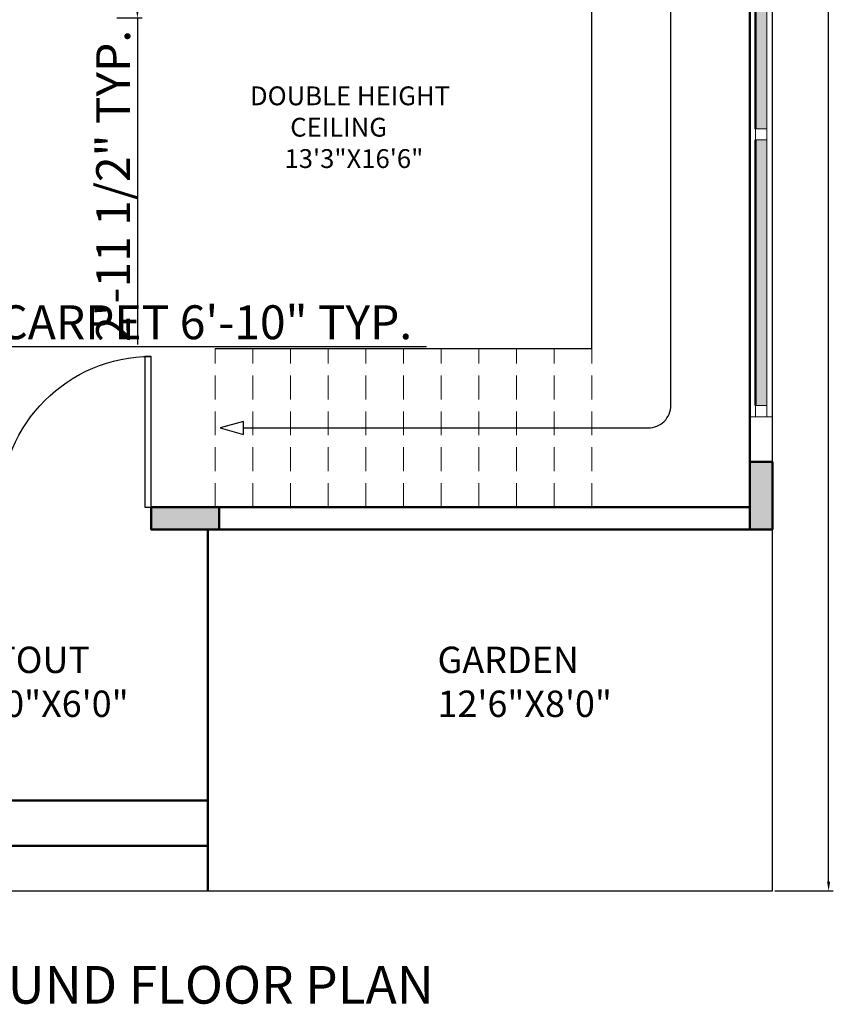
# Model space of a CAD drawing. Units: inches. Extents: x 3064 to 19385, y 846 to 15425.
# Tile 2 of 108: x 3363 to 3579, y 850 to 1112. Entities that reach past the tile are written whole.
import ezdxf

# ---------------------------------------------------------------- set-up
doc = ezdxf.new("R2010")
doc.units = ezdxf.units.IN
doc.linetypes.add('DASHED', pattern=[19.05, 12.7, -6.35])
for name, color, linetype, lineweight in [('A-ANNO-DIMS', 2, 'Continuous', 18), ('A-ANNO-TEXT', 7, 'Continuous', 25), ('A-AREA-IDEN', 3, 'Continuous', 18), ('A-COLS', 1, 'Continuous', 35), ('A-DOOR', 3, 'Continuous', 25), ('A-FLOR-STRS', 2, 'Continuous', 25), ('A-FLOR-STRS-OVHD', 2, 'DASHED', 18), ('A-GLAZ', 4, 'Continuous', 18), ('A-WALL', 7, 'Continuous', 50), ('C-PROP', 6, 'Continuous', 25)]:
    doc.layers.add(name, color=color, linetype=linetype, lineweight=lineweight)
doc.styles.get("Standard").update_dxf_attribs({"font": 'arial.ttf'})
doc.dimstyles.new('ISO-25', dxfattribs={"dimtxt": 9, "dimasz": 2.5, "dimexe": 1.25, "dimexo": 0.625, "dimtad": 1, "dimdec": 1, "dimlunit": 3, "dimtxsty": 'Standard', "dimcen": 2.5, "dimadec": 0, "dimazin": 0, "dimtfac": 1, "dimtdec": 1, "dimtmove": 0, "dimatfit": 3, "dimfxl": 1, "dimarcsym": 0})

# ---------------------------------------------------------------- blocks, each defined once
blk = doc.blocks.new('*U2')
for p, q in [((0, 0), (0, -6)), ((40, 0), (40, -6))]:
    blk.add_line(p, q)
blk.add_lwpolyline([(0, 0), (0, 40), (1.75, 40), (1.75, 0)], close=True)
blk.add_arc((0, 0), 40, 0, 90)
blk = doc.blocks.new('*D42')
at = {"layer": 'A-ANNO-DIMS', "color": 0, "lineweight": -2, "transparency": 16777216}
for p, q in [((3563.47, 1396.34), (3579.02, 1396.34)), ((3577.77, 882.84), (3577.77, 1393.84)), ((3563.47, 880.34), (3579.02, 880.34))]:
    blk.add_line(p, q, dxfattribs=at)
at = {"layer": 'A-ANNO-DIMS', "color": 0, "transparency": 16777216}
for points in [[(3577.35, 1393.84), (3578.19, 1393.84), (3577.77, 1396.34)], [(3577.35, 882.84), (3578.19, 882.84), (3577.77, 880.34)]]:
    blk.add_solid(points, dxfattribs=at)
at = {"layer": 'Defpoints', "color": 0, "transparency": 16777216}
for p in [(3562.85, 1396.34), (3577.77, 1396.34), (3562.85, 880.34)]:
    blk.add_point(p, dxfattribs=at)
at = {"layer": 'A-ANNO-DIMS', "color": 0, "transparency": 16777216, "insert": (3572.55, 1138.34), "char_height": 9, "attachment_point": 5, "rotation": 90}
blk.add_mtext("43'", dxfattribs=at)
blk = doc.blocks.new('WIN-1800-PAIR')
h = blk.add_hatch(color=256)
h.dxf.hatch_style = 1
h.paths.add_polyline_path([(0, 0), (3, 0), (3, 70.5), (0, 70.5)])
h.paths.add_polyline_path([(3, 144), (0, 144), (0, 73.5), (3, 73.5)])
blk.add_line((3, 144), (3, 73.5))
blk.add_lwpolyline([(3, 144), (0, 144), (0, 147), (3, 147)], close=True)
blk = doc.blocks.new('WIN-2000')
blk.add_line((3, 0), (3, 70.5))
blk.add_lwpolyline([(3, 70.5), (0, 70.5), (0, 73.5), (3, 73.5)], close=True)
blk = doc.blocks.new('*D415')
at = {"layer": 'A-ANNO-DIMS', "color": 0, "lineweight": -2, "transparency": 16777216}
for p, q in [((3269.07, 1036.63), (3269.07, 1023.73)), ((3350.94, 1036.63), (3350.94, 1023.73)), ((3271.57, 1024.98), (3348.44, 1024.98)), ((3350.94, 1024.98), (3470.93, 1024.98))]:
    blk.add_line(p, q, dxfattribs=at)
at = {"layer": 'A-ANNO-DIMS', "color": 0, "transparency": 16777216}
for points in [[(3271.57, 1025.39), (3271.57, 1024.56), (3269.07, 1024.98)], [(3348.44, 1025.39), (3348.44, 1024.56), (3350.94, 1024.98)]]:
    blk.add_solid(points, dxfattribs=at)
at = {"layer": 'Defpoints', "color": 0, "transparency": 16777216}
for p in [(3269.07, 1037.26), (3350.94, 1037.26), (3350.94, 1024.98)]:
    blk.add_point(p, dxfattribs=at)
at = {"layer": 'A-ANNO-DIMS', "color": 0, "transparency": 16777216, "insert": (3412.18, 1030.26), "char_height": 9, "attachment_point": 5}
blk.add_mtext('CARPET 6\'-10" TYP.', dxfattribs=at)
blk = doc.blocks.new('*D422')
at = {"layer": 'A-ANNO-DIMS', "color": 0, "lineweight": -2, "transparency": 16777216}
for p, q in [((3388.68, 1147.59), (3395.41, 1147.59)), ((3394.16, 1145.09), (3394.16, 1114.76)), ((3388.68, 1112.26), (3395.41, 1112.26)), ((3394.16, 1112.26), (3394.16, 1025.53))]:
    blk.add_line(p, q, dxfattribs=at)
at = {"layer": 'A-ANNO-DIMS', "color": 0, "transparency": 16777216}
for points in [[(3393.74, 1145.09), (3394.57, 1145.09), (3394.16, 1147.59)], [(3393.74, 1114.76), (3394.57, 1114.76), (3394.16, 1112.26)]]:
    blk.add_solid(points, dxfattribs=at)
at = {"layer": 'Defpoints', "color": 0, "transparency": 16777216}
for p in [(3388.05, 1147.59), (3388.05, 1112.26), (3394.16, 1112.26)]:
    blk.add_point(p, dxfattribs=at)
at = {"layer": 'A-ANNO-DIMS', "color": 0, "transparency": 16777216, "insert": (3388.88, 1067.64), "char_height": 9, "attachment_point": 5, "rotation": 90}
blk.add_mtext('2\'-11 1/2" TYP.', dxfattribs=at)

msp = doc.modelspace()

# ---------------------------------------------------------------- hatches: boundary and pattern name
at = {"layer": 'A-COLS'}
h = msp.add_hatch(color=256, dxfattribs=at)
h.dxf.hatch_style = 1
h.paths.add_polyline_path([(3556.85, 976.34), (3562.85, 976.34), (3562.85, 994.34), (3556.85, 994.34)])
h = msp.add_hatch(color=256, dxfattribs=at)
h.dxf.hatch_style = 1
h.paths.add_polyline_path([(3415.85, 976.34), (3415.85, 982.34), (3397.85, 982.34), (3397.85, 976.34)])

# ---------------------------------------------------------------- linework, layer by layer
at = {"layer": 'A-FLOR-STRS'}
for q in [(3514.85, 1180.34), (3414.85, 1024.34)]:
    msp.add_line((3514.85, 1024.34), q, dxfattribs=at)
msp.add_lwpolyline([(3422.34, 1003.34), (3529.85, 1003.34, 0.414214), (3535.85, 1009.34), (3535.85, 1153.34, 0.414214), (3529.85, 1159.34), (3402.85, 1159.34)], format="xyb", dxfattribs=at)
msp.add_lwpolyline([(3416.14, 1003.34), (3422.34, 1001.61), (3422.34, 1005.07)], close=True, dxfattribs=at)
at = {"layer": 'A-FLOR-STRS-OVHD', "ltscale": 0.5}
for p, q in [((3414.85, 982.34), (3414.85, 1024.34)), ((3424.85, 982.34), (3424.85, 1024.34)), ((3434.85, 982.34), (3434.85, 1024.34)), ((3444.85, 982.34), (3444.85, 1024.34)), ((3454.85, 982.34), (3454.85, 1024.34)), ((3464.85, 982.34), (3464.85, 1024.34)), ((3474.85, 982.34), (3474.85, 1024.34)), ((3484.85, 982.34), (3484.85, 1024.34)), ((3494.85, 982.34), (3494.85, 1024.34)), ((3504.85, 982.34), (3504.85, 1024.34)), ((3514.85, 982.34), (3514.85, 1024.34))]:
    msp.add_line(p, q, dxfattribs=at)
at = {"layer": 'A-GLAZ'}
msp.add_line((3562.85, 1006.34), (3556.85, 1006.34), dxfattribs=at)
msp.add_line((3562.85, 1006.34), (3556.85, 1006.34), dxfattribs=at)
msp.add_lwpolyline([(3561.35, 1006.34), (3558.35, 1006.34), (3558.35, 1009.34), (3561.35, 1009.34)], close=True, dxfattribs=at)
at = {"layer": 'A-WALL'}
for p, q in [((3556.85, 982.34), (3556.85, 1180.34)), ((3558.35, 1153.34), (3558.35, 1082.84)), ((3558.35, 1009.34), (3558.35, 1079.84)), ((3556.85, 982.34), (3397.85, 982.34)), ((3397.85, 976.34), (3397.85, 982.34)), ((3562.85, 976.34), (3397.85, 976.34)), ((3412.85, 976.34), (3412.85, 880.34)), ((3220.85, 904.34), (3412.85, 904.34)), ((3220.85, 892.34), (3412.85, 892.34))]:
    msp.add_line(p, q, dxfattribs=at)
for points in [[(3562.85, 976.34), (3562.85, 994.34), (3556.85, 994.34), (3556.85, 976.34)], [(3415.85, 982.34), (3397.85, 982.34), (3397.85, 976.34), (3415.85, 976.34)]]:
    msp.add_lwpolyline(points, close=True, dxfattribs=at)
at = {"layer": 'C-PROP'}
for p, q in [((3562.85, 880.34), (3562.85, 1396.34)), ((3220.85, 880.34), (3562.85, 880.34))]:
    msp.add_line(p, q, dxfattribs=at)

# ---------------------------------------------------------------- block references
at = {"layer": 'A-DOOR', "xscale": -1}
msp.add_blockref('*U2', (3397.85, 982.34), dxfattribs=at)
at = {"layer": 'A-GLAZ'}
for name in ['WIN-1800-PAIR', 'WIN-2000']:
    msp.add_blockref(name, (3558.35, 1009.34), dxfattribs=at)

# ---------------------------------------------------------------- texts
at = {"layer": 'A-ANNO-TEXT', "insert": (3331.51, 860.41), "char_height": 10, "attachment_point": 1}
msp.add_mtext_dynamic_manual_height_columns('GROUND FLOOR PLAN', width=200.9739, gutter_width=12.5, heights=[0], dxfattribs=at)
at = {"layer": 'A-AREA-IDEN', "attachment_point": 1}
for s, width, insert, char_height in [('DOUBLE HEIGHT \\P       CEILING            \\P      13\'3"X16\'6"', 57.0817, (3424.06, 1094.07), 5), (' SITOUT\\P16\'0"X6\'0"', 67.5924, (3345.51, 945.24), 7), ('GARDEN\\P12\'6"X8\'0"', 67.5924, (3473.89, 945.24), 7)]:
    msp.add_mtext_dynamic_manual_height_columns(s, width=width, gutter_width=12.5, heights=[0], dxfattribs=dict(at, insert=insert, char_height=char_height))

# ---------------------------------------------------------------- dimensions: what is measured, and where the dimension line sits
at = {"layer": 'A-ANNO-DIMS'}
dim = msp.add_linear_dim(base=(3577.77, 1396.34), p1=(3562.85, 880.34), p2=(3562.85, 1396.34), angle=90, dimstyle='ISO-25', override={"dimclrd": 0, "dimclre": 0, "dimclrt": 0}, dxfattribs=at)
dim.commit()
dim.dimension.update_dxf_attribs({"geometry": '*D42', "text_midpoint": (3572.55, 1138.34)})
dim = msp.add_linear_dim(base=(3394.16, 1112.26), p1=(3388.05, 1147.59), p2=(3388.05, 1112.26), angle=270, text='<> TYP.', dimstyle='ISO-25', override={"dimdec": 1, "dimrnd": 0, "dimzin": 1, "dimlunit": 4, "dimfrac": 2}, dxfattribs=at)
dim.commit()
dim.dimension.update_dxf_attribs({"geometry": '*D422', "text_midpoint": (3388.88, 1067.64)})
dim = msp.add_linear_dim(base=(3350.94, 1024.98), p1=(3269.07, 1037.26), p2=(3350.94, 1037.26), text='CARPET <> TYP.', dimstyle='ISO-25', override={"dimdec": 1, "dimrnd": 0, "dimzin": 1, "dimlunit": 4, "dimfrac": 2}, dxfattribs=at)
dim.commit()
dim.dimension.update_dxf_attribs({"geometry": '*D415', "text_midpoint": (3412.18, 1030.26)})

doc.saveas('drawing.dxf')
